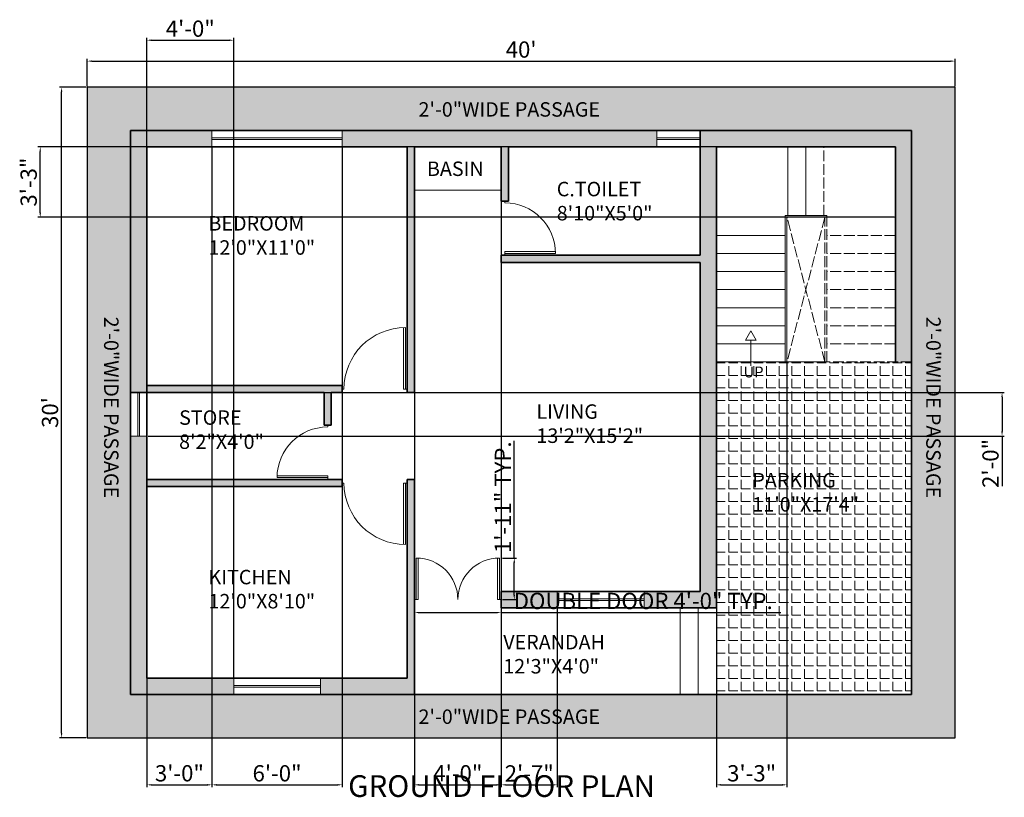
# Model space of a CAD drawing. Units: inches. Extents: x 1947 to 4744, y 610 to 1869.
# Tile 2 of 8: x 1947 to 2492, y 1428 to 1858. Entities that reach past the tile are written whole.
import ezdxf

# ---------------------------------------------------------------- set-up
doc = ezdxf.new("R2010")
doc.units = ezdxf.units.IN
doc.linetypes.add('ACAD_ISO02W100', pattern=[15, 12, -3])
for name, color, linetype, lineweight in [('A-ANNO-DIMS', 2, 'Continuous', 18), ('A-ANNO-SYMB', 2, 'Continuous', 18), ('A-ANNO-TEXT', 7, 'Continuous', 18), ('A-ANNO-TITL', 7, 'Continuous', 35), ('A-AREA-IDEN', 7, 'Continuous', 18), ('A-DOOR', 3, 'Continuous', 18), ('A-FLOR-FIXT', 9, 'Continuous', 18), ('A-FLOR-STRS', 7, 'Continuous', 18), ('A-FLOR-STRS-OVHD', 7, 'ACAD_ISO02W100', 13), ('A-GLAZ', 4, 'Continuous', 18), ('A-WALL', 7, 'Continuous', 35), ('C-PROP', 8, 'Continuous', 25)]:
    doc.layers.add(name, color=color, linetype=linetype, lineweight=lineweight)
doc.layers.add('A-FLOR-PATT', color=251, linetype='Continuous', lineweight=13, true_color=0x636466)
doc.layers.add('A-WALL-PATT', color=18, linetype='Continuous', lineweight=13, true_color=0x000000)
doc.styles.get("Standard").update_dxf_attribs({"font": 'arial.ttf'})
doc.dimstyles.new('ISO-25', dxfattribs={"dimtxt": 9, "dimasz": 2.5, "dimexe": 1.25, "dimexo": 0.625, "dimtad": 1, "dimdec": 1, "dimlunit": 3, "dimtxsty": 'Standard', "dimcen": 2.5, "dimadec": 0, "dimazin": 0, "dimtfac": 1, "dimtdec": 1, "dimtmove": 0, "dimatfit": 3, "dimfxl": 1, "dimarcsym": 0})
pattern_1 = [(0, (-1704.723, -21.7476), (0, 6.985), [5.08, -1.905]), (90, (-1704.723, -21.7476), (-6.985, 4e-16), [5.08, -1.905])]

# ---------------------------------------------------------------- blocks, each defined once
blk = doc.blocks.new('1')
for p, q in [((4267.36, 1627.82), (4267.36, 1650.82)), ((4268.36, 1627.82), (4268.36, 1650.82)), ((4312.36, 1627.82), (4312.36, 1650.82)), ((4313.36, 1627.82), (4313.36, 1650.82)), ((4266.36, 1627.82), (4268.36, 1627.82)), ((4314.36, 1627.82), (4312.36, 1627.82))]:
    blk.add_line(p, q)
at = {"ltscale": 0.5}
for centre, start, end in [((4267.36, 1627.82), 0, 90), ((4313.36, 1627.82), 90, 180)]:
    blk.add_arc(centre, 23, start, end, dxfattribs=at)
blk = doc.blocks.new('2')
for p, q in [((4319.45, 1679.18), (4319.45, 1713.18)), ((4320.45, 1679.18), (4320.45, 1713.18)), ((4318.45, 1679.18), (4320.45, 1679.18)), ((4353.45, 1679.18), (4354.45, 1679.18))]:
    blk.add_line(p, q)
at = {"ltscale": 0.5}
blk.add_arc((4319.45, 1679.18), 34, 0, 90, dxfattribs=at)
blk = doc.blocks.new('4')
for p, q in [((3808.6, 1693.11), (3808.6, 1721.11)), ((3809.6, 1693.11), (3809.6, 1721.11)), ((3807.6, 1693.11), (3809.6, 1693.11)), ((3836.6, 1693.11), (3837.6, 1693.11))]:
    blk.add_line(p, q)
at = {"ltscale": 0.5}
blk.add_arc((3808.6, 1693.11), 28, 0, 90, dxfattribs=at)
blk = doc.blocks.new('*D64')
at = {"layer": 'A-ANNO-DIMS', "color": 0, "lineweight": -2, "transparency": 16777216}
for p, q in [((1984.18, 1821.08), (1969.39, 1821.08)), ((1970.64, 1463.58), (1970.64, 1818.58)), ((1984.18, 1461.08), (1969.39, 1461.08))]:
    blk.add_line(p, q, dxfattribs=at)
at = {"layer": 'A-ANNO-DIMS', "color": 0, "transparency": 16777216}
for points in [[(1970.22, 1818.58), (1971.05, 1818.58), (1970.64, 1821.08)], [(1970.22, 1463.58), (1971.05, 1463.58), (1970.64, 1461.08)]]:
    blk.add_solid(points, dxfattribs=at)
at = {"layer": 'Defpoints', "color": 0, "transparency": 16777216}
for p in [(1970.64, 1821.08), (1984.81, 1821.08), (1984.81, 1461.08)]:
    blk.add_point(p, dxfattribs=at)
at = {"layer": 'A-ANNO-DIMS', "color": 0, "transparency": 16777216, "insert": (1965.41, 1641.08), "char_height": 9, "attachment_point": 5, "rotation": 90}
blk.add_mtext("30'", dxfattribs=at)
blk = doc.blocks.new('*D65')
at = {"layer": 'A-ANNO-DIMS', "color": 0, "lineweight": -2, "transparency": 16777216}
for p, q in [((1984.81, 1821.71), (1984.81, 1836.77)), ((1987.31, 1835.52), (2462.31, 1835.52)), ((2464.81, 1821.71), (2464.81, 1836.77))]:
    blk.add_line(p, q, dxfattribs=at)
at = {"layer": 'A-ANNO-DIMS', "color": 0, "transparency": 16777216}
for points in [[(1987.31, 1835.93), (1987.31, 1835.1), (1984.81, 1835.52)], [(2462.31, 1835.93), (2462.31, 1835.1), (2464.81, 1835.52)]]:
    blk.add_solid(points, dxfattribs=at)
at = {"layer": 'Defpoints', "color": 0, "transparency": 16777216}
for p in [(2464.81, 1835.52), (1984.81, 1821.08), (2464.81, 1821.08)]:
    blk.add_point(p, dxfattribs=at)
at = {"layer": 'A-ANNO-DIMS', "color": 0, "transparency": 16777216, "insert": (2224.81, 1840.74), "char_height": 9, "attachment_point": 5}
blk.add_mtext("40'", dxfattribs=at)
blk = doc.blocks.new('STAIR-DIRECTION')
blk.add_line((2.91, 14.18), (2.91, 0))
blk.add_lwpolyline([(2.91, 19.23), (0, 14.18), (5.83, 14.18)], close=True)
blk = doc.blocks.new('*D78')
at = {"layer": 'A-ANNO-DIMS', "color": 0, "lineweight": -2, "transparency": 16777216}
for p, q in [((2165.81, 1536.96), (2165.81, 1529.13)), ((2213.81, 1536.96), (2213.81, 1529.13)), ((2168.31, 1530.38), (2211.31, 1530.38)), ((2213.81, 1530.38), (2368.38, 1530.38))]:
    blk.add_line(p, q, dxfattribs=at)
at = {"layer": 'A-ANNO-DIMS', "color": 0, "transparency": 16777216}
for points in [[(2168.31, 1530.8), (2168.31, 1529.96), (2165.81, 1530.38)], [(2211.31, 1530.8), (2211.31, 1529.96), (2213.81, 1530.38)]]:
    blk.add_solid(points, dxfattribs=at)
at = {"layer": 'Defpoints', "color": 0, "transparency": 16777216}
for p in [(2165.81, 1537.58), (2213.81, 1537.58), (2213.81, 1530.38)]:
    blk.add_point(p, dxfattribs=at)
at = {"layer": 'A-ANNO-DIMS', "color": 0, "transparency": 16777216, "insert": (2292.34, 1535.66), "char_height": 9, "attachment_point": 5}
blk.add_mtext('DOUBLE DOOR 4\'-0" TYP.', dxfattribs=at)
blk = doc.blocks.new('*D79')
at = {"layer": 'A-ANNO-DIMS', "color": 0, "lineweight": -2, "transparency": 16777216}
for p, q in [((2221.01, 1560.58), (2221.01, 1625.33)), ((2214.43, 1560.58), (2222.26, 1560.58)), ((2221.01, 1540.08), (2221.01, 1558.08)), ((2214.43, 1537.58), (2222.26, 1537.58))]:
    blk.add_line(p, q, dxfattribs=at)
at = {"layer": 'A-ANNO-DIMS', "color": 0, "transparency": 16777216}
for points in [[(2220.59, 1558.08), (2221.42, 1558.08), (2221.01, 1560.58)], [(2220.59, 1540.08), (2221.42, 1540.08), (2221.01, 1537.58)]]:
    blk.add_solid(points, dxfattribs=at)
at = {"layer": 'Defpoints', "color": 0, "transparency": 16777216}
for p in [(2213.81, 1560.58), (2221.01, 1560.58), (2213.81, 1537.58)]:
    blk.add_point(p, dxfattribs=at)
at = {"layer": 'A-ANNO-DIMS', "color": 0, "transparency": 16777216, "insert": (2215.86, 1594.21), "char_height": 9, "attachment_point": 5, "rotation": 90}
blk.add_mtext('1\'-11" TYP.', dxfattribs=at)
blk = doc.blocks.new('*D96')
at = {"layer": 'A-ANNO-DIMS', "color": 0, "lineweight": -2, "transparency": 16777216}
for p, q in [((2332.81, 1668.46), (2332.81, 1433.83)), ((2371.81, 1668.46), (2371.81, 1433.83)), ((2335.31, 1435.08), (2369.31, 1435.08))]:
    blk.add_line(p, q, dxfattribs=at)
at = {"layer": 'A-ANNO-DIMS', "color": 0, "transparency": 16777216}
for points in [[(2335.31, 1435.5), (2335.31, 1434.66), (2332.81, 1435.08)], [(2369.31, 1435.5), (2369.31, 1434.66), (2371.81, 1435.08)]]:
    blk.add_solid(points, dxfattribs=at)
at = {"layer": 'Defpoints', "color": 0, "transparency": 16777216}
for p in [(2332.81, 1669.08), (2371.81, 1669.08), (2371.81, 1435.08)]:
    blk.add_point(p, dxfattribs=at)
at = {"layer": 'A-ANNO-DIMS', "color": 0, "transparency": 16777216, "insert": (2352.31, 1440.3), "char_height": 9, "attachment_point": 5}
blk.add_mtext('3\'-3"', dxfattribs=at)
blk = doc.blocks.new('*D97')
at = {"layer": 'A-ANNO-DIMS', "color": 0, "lineweight": -2, "transparency": 16777216}
for p, q in [((2431.18, 1788.08), (1957.56, 1788.08)), ((1958.81, 1751.58), (1958.81, 1785.58)), ((2431.18, 1749.08), (1957.56, 1749.08))]:
    blk.add_line(p, q, dxfattribs=at)
at = {"layer": 'A-ANNO-DIMS', "color": 0, "transparency": 16777216}
for points in [[(1958.39, 1785.58), (1959.22, 1785.58), (1958.81, 1788.08)], [(1958.39, 1751.58), (1959.22, 1751.58), (1958.81, 1749.08)]]:
    blk.add_solid(points, dxfattribs=at)
at = {"layer": 'Defpoints', "color": 0, "transparency": 16777216}
for p in [(1958.81, 1788.08), (2431.81, 1788.08), (2431.81, 1749.08)]:
    blk.add_point(p, dxfattribs=at)
at = {"layer": 'A-ANNO-DIMS', "color": 0, "transparency": 16777216, "insert": (1953.58, 1768.58), "char_height": 9, "attachment_point": 5, "rotation": 90}
blk.add_mtext('3\'-3"', dxfattribs=at)
blk = doc.blocks.new('*D99')
at = {"layer": 'A-ANNO-DIMS', "color": 0, "lineweight": -2, "transparency": 16777216}
for p, q in [((2165.81, 1763.46), (2165.81, 1433.83)), ((2213.81, 1763.46), (2213.81, 1433.83)), ((2168.31, 1435.08), (2211.31, 1435.08))]:
    blk.add_line(p, q, dxfattribs=at)
at = {"layer": 'A-ANNO-DIMS', "color": 0, "transparency": 16777216}
for points in [[(2168.31, 1435.5), (2168.31, 1434.66), (2165.81, 1435.08)], [(2211.31, 1435.5), (2211.31, 1434.66), (2213.81, 1435.08)]]:
    blk.add_solid(points, dxfattribs=at)
at = {"layer": 'Defpoints', "color": 0, "transparency": 16777216}
for p in [(2165.81, 1764.08), (2213.81, 1764.08), (2213.81, 1435.08)]:
    blk.add_point(p, dxfattribs=at)
at = {"layer": 'A-ANNO-DIMS', "color": 0, "transparency": 16777216, "insert": (2189.81, 1440.3), "char_height": 9, "attachment_point": 5}
blk.add_mtext('4\'-0"', dxfattribs=at)
blk = doc.blocks.new('*D104')
at = {"layer": 'A-ANNO-DIMS', "color": 0, "lineweight": -2, "transparency": 16777216}
for p, q in [((2017.81, 1787.46), (2017.81, 1433.83)), ((2053.81, 1787.46), (2053.81, 1433.83)), ((2020.31, 1435.08), (2051.31, 1435.08))]:
    blk.add_line(p, q, dxfattribs=at)
at = {"layer": 'A-ANNO-DIMS', "color": 0, "transparency": 16777216}
for points in [[(2020.31, 1435.5), (2020.31, 1434.66), (2017.81, 1435.08)], [(2051.31, 1435.5), (2051.31, 1434.66), (2053.81, 1435.08)]]:
    blk.add_solid(points, dxfattribs=at)
at = {"layer": 'Defpoints', "color": 0, "transparency": 16777216}
for p in [(2017.81, 1788.08), (2053.81, 1788.08), (2053.81, 1435.08)]:
    blk.add_point(p, dxfattribs=at)
at = {"layer": 'A-ANNO-DIMS', "color": 0, "transparency": 16777216, "insert": (2035.81, 1440.3), "char_height": 9, "attachment_point": 5}
blk.add_mtext('3\'-0"', dxfattribs=at)
blk = doc.blocks.new('*D105')
at = {"layer": 'A-ANNO-DIMS', "color": 0, "lineweight": -2, "transparency": 16777216}
for p, q in [((2053.81, 1787.46), (2053.81, 1433.83)), ((2125.81, 1787.46), (2125.81, 1433.83)), ((2056.31, 1435.08), (2123.31, 1435.08))]:
    blk.add_line(p, q, dxfattribs=at)
at = {"layer": 'A-ANNO-DIMS', "color": 0, "transparency": 16777216}
for points in [[(2056.31, 1435.5), (2056.31, 1434.66), (2053.81, 1435.08)], [(2123.31, 1435.5), (2123.31, 1434.66), (2125.81, 1435.08)]]:
    blk.add_solid(points, dxfattribs=at)
at = {"layer": 'Defpoints', "color": 0, "transparency": 16777216}
for p in [(2053.81, 1788.08), (2125.81, 1788.08), (2125.81, 1435.08)]:
    blk.add_point(p, dxfattribs=at)
at = {"layer": 'A-ANNO-DIMS', "color": 0, "transparency": 16777216, "insert": (2089.81, 1440.3), "char_height": 9, "attachment_point": 5}
blk.add_mtext('6\'-0"', dxfattribs=at)
blk = doc.blocks.new('*D106')
at = {"layer": 'A-ANNO-DIMS', "color": 0, "lineweight": -2, "transparency": 16777216}
for p, q in [((2017.81, 1494.71), (2017.81, 1848.33)), ((2020.31, 1847.08), (2063.31, 1847.08)), ((2065.81, 1494.71), (2065.81, 1848.33))]:
    blk.add_line(p, q, dxfattribs=at)
at = {"layer": 'A-ANNO-DIMS', "color": 0, "transparency": 16777216}
for points in [[(2020.31, 1847.5), (2020.31, 1846.66), (2017.81, 1847.08)], [(2063.31, 1847.5), (2063.31, 1846.66), (2065.81, 1847.08)]]:
    blk.add_solid(points, dxfattribs=at)
at = {"layer": 'Defpoints', "color": 0, "transparency": 16777216}
for p in [(2065.81, 1847.08), (2017.81, 1494.08), (2065.81, 1494.08)]:
    blk.add_point(p, dxfattribs=at)
at = {"layer": 'A-ANNO-DIMS', "color": 0, "transparency": 16777216, "insert": (2041.81, 1852.3), "char_height": 9, "attachment_point": 5}
blk.add_mtext('4\'-0"', dxfattribs=at)
blk = doc.blocks.new('*D107')
at = {"layer": 'A-ANNO-DIMS', "color": 0, "lineweight": -2, "transparency": 16777216}
for p, q in [((2213.81, 1532.46), (2213.81, 1433.83)), ((2244.81, 1532.46), (2244.81, 1433.83)), ((2216.31, 1435.08), (2242.31, 1435.08))]:
    blk.add_line(p, q, dxfattribs=at)
at = {"layer": 'A-ANNO-DIMS', "color": 0, "transparency": 16777216}
for points in [[(2216.31, 1435.5), (2216.31, 1434.66), (2213.81, 1435.08)], [(2242.31, 1435.5), (2242.31, 1434.66), (2244.81, 1435.08)]]:
    blk.add_solid(points, dxfattribs=at)
at = {"layer": 'Defpoints', "color": 0, "transparency": 16777216}
for p in [(2213.81, 1533.08), (2244.81, 1533.08), (2244.81, 1435.08)]:
    blk.add_point(p, dxfattribs=at)
at = {"layer": 'A-ANNO-DIMS', "color": 0, "transparency": 16777216, "insert": (2229.31, 1440.22), "char_height": 9, "attachment_point": 5}
blk.add_mtext('2\'-7"', dxfattribs=at)
blk = doc.blocks.new('*D111')
at = {"layer": 'A-ANNO-DIMS', "color": 0, "lineweight": -2, "transparency": 16777216}
for p, q in [((2018.43, 1652.08), (2492.06, 1652.08)), ((2490.81, 1649.58), (2490.81, 1630.58)), ((2018.43, 1628.08), (2492.06, 1628.08)), ((2490.81, 1628.08), (2490.81, 1600.25))]:
    blk.add_line(p, q, dxfattribs=at)
at = {"layer": 'A-ANNO-DIMS', "color": 0, "transparency": 16777216}
for points in [[(2490.39, 1649.58), (2491.22, 1649.58), (2490.81, 1652.08)], [(2490.39, 1630.58), (2491.22, 1630.58), (2490.81, 1628.08)]]:
    blk.add_solid(points, dxfattribs=at)
at = {"layer": 'Defpoints', "color": 0, "transparency": 16777216}
for p in [(2017.81, 1652.08), (2017.81, 1628.08), (2490.81, 1628.08)]:
    blk.add_point(p, dxfattribs=at)
at = {"layer": 'A-ANNO-DIMS', "color": 0, "transparency": 16777216, "insert": (2485.59, 1612.92), "char_height": 9, "attachment_point": 5, "rotation": 90}
blk.add_mtext('2\'-0"', dxfattribs=at)

msp = doc.modelspace()

# ---------------------------------------------------------------- hatches: boundary and pattern name
at = {"layer": 'A-FLOR-PATT'}
h = msp.add_hatch(dxfattribs=at)
h.set_pattern_fill('ANGLE', color=256)
h.set_pattern_definition(pattern_1)
h.paths.add_polyline_path([(1984.81, 1821.08), (1984.81, 1461.08), (2464.81, 1461.08), (2464.81, 1821.08)])
h.paths.add_polyline_path([(2440.81, 1797.08), (2440.81, 1485.08), (2008.81, 1485.08), (2008.81, 1797.08)], flags=16)
h.paths.add_polyline_path([(2431.81, 1788.08), (2431.81, 1669.08), (2392.81, 1669.08), (2332.81, 1669.08), (2332.81, 1533.08), (2213.81, 1533.08), (2213.81, 1542.08), (2323.81, 1542.08), (2323.81, 1724.08), (2213.81, 1724.08), (2213.81, 1728.08), (2323.81, 1728.08), (2323.81, 1788.08), (2217.81, 1788.08), (2217.81, 1758.08), (2213.81, 1758.08), (2213.81, 1764.08), (2165.81, 1764.08), (2165.81, 1652.08), (2161.81, 1652.08), (2161.81, 1788.08), (2017.81, 1788.08), (2017.81, 1656.08), (2125.81, 1656.08), (2125.81, 1652.08), (2119.81, 1652.08), (2119.81, 1634.08), (2115.81, 1634.08), (2115.81, 1652.08), (2017.81, 1652.08), (2017.81, 1604.08), (2125.81, 1604.08), (2125.81, 1600.08), (2017.81, 1600.08), (2017.81, 1494.08), (2113.81, 1494.08), (2113.81, 1489.08), (2065.81, 1489.08), (2065.81, 1494.08), (2017.81, 1494.08), (2017.81, 1600.08), (2125.81, 1600.08), (2125.81, 1604.08), (2017.81, 1604.08), (2017.81, 1628.08), (2012.81, 1628.08), (2012.81, 1652.08), (2115.81, 1652.08), (2115.81, 1634.08), (2119.81, 1634.08), (2119.81, 1652.08), (2125.81, 1652.08), (2125.81, 1656.08), (2017.81, 1656.08), (2017.81, 1788.08), (2053.81, 1788.08), (2053.81, 1793.08), (2125.81, 1793.08), (2125.81, 1788.08), (2161.81, 1788.08), (2161.81, 1652.08), (2165.81, 1652.08), (2165.81, 1788.08), (2213.81, 1788.08), (2213.81, 1758.08), (2217.81, 1758.08), (2217.81, 1788.08), (2299.81, 1788.08), (2299.81, 1793.08), (2323.81, 1793.08), (2323.81, 1728.08), (2213.81, 1728.08), (2213.81, 1724.08), (2323.81, 1724.08), (2323.81, 1542.08), (2292.81, 1542.08), (2292.81, 1533.08), (2332.81, 1533.08), (2332.81, 1788.08)], flags=0)
h.paths.add_polyline_path([(2371.81, 1749.08), (2392.81, 1749.08), (2392.81, 1669.08), (2382.31, 1709.08), (2371.81, 1669.08)], flags=0)
h.paths.add_polyline_path([(2170.5, 1767.41), (2209.94, 1767.41), (2209.94, 1784.49), (2170.5, 1784.49)], flags=8)
h.paths.add_polyline_path([(2165.8, 1464.23), (2278.79, 1464.23), (2278.79, 1481.31), (2165.8, 1481.31)], flags=24)
h.paths.add_polyline_path([(1989.56, 1696.36), (1989.56, 1583.37), (2006.64, 1583.37), (2006.64, 1696.36)], flags=24)
h.paths.add_polyline_path([(2444.3, 1696.36), (2444.3, 1583.37), (2461.38, 1583.37), (2461.38, 1696.36)], flags=24)
h.paths.add_polyline_path([(2165.8, 1800.23), (2278.79, 1800.23), (2278.79, 1817.31), (2165.8, 1817.31)], flags=24)
h.paths.add_polyline_path([(2211.53, 1492.13), (2283.09, 1492.13), (2283.09, 1522.55), (2211.53, 1522.55)], flags=8)
h.paths.add_polyline_path([(2349.32, 1581.74), (2411.18, 1581.74), (2411.18, 1612.15), (2349.32, 1612.15)], flags=8)
h.paths.add_polyline_path([(2032.89, 1616.39), (2082.97, 1616.39), (2082.97, 1646.8), (2032.89, 1646.8)], flags=8)
h.paths.add_polyline_path([(2241.79, 1742.83), (2298.24, 1742.83), (2298.24, 1773.25), (2241.79, 1773.25)], flags=8)
h.paths.add_polyline_path([(2229.87, 1619.7), (2291.74, 1619.7), (2291.74, 1650.11), (2229.87, 1650.11)], flags=8)
h.paths.add_polyline_path([(2048.47, 1528.14), (2110.34, 1528.14), (2110.34, 1558.56), (2048.47, 1558.56)], flags=8)
h.paths.add_polyline_path([(2048.47, 1723.84), (2112.73, 1723.84), (2112.73, 1754.25), (2048.47, 1754.25)], flags=8)
h = msp.add_hatch(dxfattribs=at)
h.set_pattern_fill('ANGLE', color=256)
h.set_pattern_definition(pattern_1)
h.paths.add_polyline_path([(2440.81, 1669.08), (2392.81, 1669.08), (2332.81, 1669.08), (2332.81, 1533.08), (2332.81, 1485.08), (2440.81, 1485.08)])
h.paths.add_polyline_path([(2346.28, 1657.09), (2360.6, 1657.09), (2360.6, 1669.9), (2346.28, 1669.9)], flags=9)
h.paths.add_polyline_path([(2349.32, 1581.74), (2411.18, 1581.74), (2411.18, 1612.15), (2349.32, 1612.15)], flags=24)
at = {"layer": 'A-WALL-PATT'}
h = msp.add_hatch(color=256, dxfattribs=at)
h.dxf.hatch_style = 1
h.paths.add_polyline_path([(2053.81, 1788.08), (2053.81, 1797.08), (2008.81, 1797.08), (2008.81, 1652.08), (2115.81, 1652.08), (2115.81, 1634.08), (2119.81, 1634.08), (2119.81, 1652.08), (2125.81, 1652.08), (2125.81, 1656.08), (2017.81, 1656.08), (2017.81, 1788.08)])
h.paths.add_polyline_path([(2125.81, 1797.08), (2125.81, 1788.08), (2161.81, 1788.08), (2161.81, 1652.08), (2165.81, 1652.08), (2165.81, 1788.08), (2213.81, 1788.08), (2213.81, 1758.08), (2217.81, 1758.08), (2217.81, 1788.08), (2299.81, 1788.08), (2299.81, 1797.08)])
h.paths.add_polyline_path([(2323.81, 1728.08), (2213.81, 1728.08), (2213.81, 1724.08), (2323.81, 1724.08), (2323.81, 1542.08), (2292.81, 1542.08), (2292.81, 1533.08), (2332.81, 1533.08), (2332.81, 1788.08), (2431.81, 1788.08), (2431.81, 1669.08), (2440.81, 1669.08), (2440.81, 1797.08), (2323.81, 1797.08)])
h.paths.add_polyline_path([(2165.81, 1485.08), (2165.81, 1604.08), (2161.81, 1604.08), (2161.81, 1494.08), (2113.81, 1494.08), (2113.81, 1485.08)])
h.paths.add_polyline_path([(2017.81, 1494.08), (2017.81, 1600.08), (2125.81, 1600.08), (2125.81, 1604.08), (2017.81, 1604.08), (2017.81, 1628.08), (2008.81, 1628.08), (2008.81, 1485.08), (2065.81, 1485.08), (2065.81, 1494.08)])
h.paths.add_polyline_path([(2244.81, 1533.08), (2244.81, 1542.08), (2213.81, 1542.08), (2213.81, 1533.08)], flags=17)

# ---------------------------------------------------------------- linework, layer by layer
at = {"layer": 'A-FLOR-FIXT'}
msp.add_line((2213.81, 1764.08), (2165.81, 1764.08), dxfattribs=at)
at = {"layer": 'A-FLOR-STRS'}
for p, q in [((2372.31, 1750.08), (2372.31, 1788.08)), ((2382.31, 1750.08), (2382.31, 1788.08)), ((2370.81, 1749.08), (2332.81, 1749.08)), ((2393.81, 1750.08), (2370.81, 1750.08)), ((2370.81, 1669.08), (2370.81, 1750.08)), ((2392.81, 1749.08), (2371.81, 1749.08)), ((2371.81, 1669.08), (2371.81, 1749.08)), ((2370.81, 1739.08), (2332.81, 1739.08)), ((2370.81, 1729.08), (2332.81, 1729.08)), ((2370.81, 1719.08), (2332.81, 1719.08)), ((2370.81, 1709.08), (2332.81, 1709.08)), ((2370.81, 1699.08), (2332.81, 1699.08)), ((2370.81, 1689.08), (2332.81, 1689.08)), ((2370.81, 1679.08), (2332.81, 1679.08)), ((2392.81, 1669.08), (2332.81, 1669.08)), ((2312.81, 1533.08), (2312.81, 1485.08)), ((2322.81, 1533.08), (2322.81, 1485.08)), ((2332.81, 1533.08), (2332.81, 1485.08))]:
    msp.add_line(p, q, dxfattribs=at)
at = {"layer": 'A-FLOR-STRS-OVHD', "ltscale": 0.5}
for p, q in [((2392.31, 1750.08), (2392.31, 1788.08)), ((2392.81, 1749.08), (2371.81, 1669.08)), ((2392.81, 1669.08), (2371.81, 1749.08)), ((2392.81, 1669.08), (2392.81, 1749.08)), ((2393.81, 1669.08), (2393.81, 1750.08)), ((2431.81, 1749.08), (2393.81, 1749.08)), ((2431.81, 1739.08), (2393.81, 1739.08)), ((2431.81, 1729.08), (2393.81, 1729.08)), ((2431.81, 1719.08), (2393.81, 1719.08)), ((2431.81, 1709.08), (2393.81, 1709.08)), ((2431.81, 1699.08), (2393.81, 1699.08)), ((2431.81, 1689.08), (2393.81, 1689.08)), ((2431.81, 1679.08), (2393.81, 1679.08)), ((2440.81, 1669.08), (2392.81, 1669.08))]:
    msp.add_line(p, q, dxfattribs=at)
at = {"layer": 'A-GLAZ'}
for p, q in [((2053.81, 1788.08), (2053.81, 1797.08)), ((2125.81, 1793.08), (2053.81, 1793.08)), ((2125.81, 1792.08), (2053.81, 1792.08)), ((2125.81, 1788.08), (2125.81, 1797.08)), ((2299.81, 1788.08), (2299.81, 1797.08)), ((2323.81, 1793.08), (2299.81, 1793.08)), ((2323.81, 1792.08), (2299.81, 1792.08)), ((2012.81, 1652.08), (2012.81, 1628.08)), ((2013.81, 1652.08), (2013.81, 1628.08)), ((2017.81, 1628.08), (2008.81, 1628.08)), ((2244.81, 1533.08), (2244.81, 1542.08)), ((2292.81, 1533.08), (2292.81, 1542.08)), ((2292.81, 1538.08), (2244.81, 1538.08)), ((2292.81, 1537.08), (2244.81, 1537.08)), ((2065.81, 1485.08), (2065.81, 1494.08)), ((2113.81, 1485.08), (2113.81, 1494.08)), ((2113.81, 1490.08), (2065.81, 1490.08)), ((2113.81, 1489.08), (2065.81, 1489.08))]:
    msp.add_line(p, q, dxfattribs=at)
at = {"layer": 'A-WALL'}
for p, q in [((2440.81, 1797.08), (2008.81, 1797.08)), ((2008.81, 1797.08), (2008.81, 1485.08)), ((2323.81, 1728.08), (2323.81, 1797.08)), ((2440.81, 1485.08), (2440.81, 1797.08)), ((2161.81, 1788.08), (2017.81, 1788.08)), ((2017.81, 1788.08), (2017.81, 1656.08)), ((2161.81, 1788.08), (2161.81, 1652.08)), ((2213.81, 1788.08), (2165.81, 1788.08)), ((2165.81, 1788.08), (2165.81, 1652.08)), ((2213.81, 1758.08), (2213.81, 1788.08)), ((2323.81, 1788.08), (2217.81, 1788.08)), ((2217.81, 1758.08), (2217.81, 1788.08)), ((2431.81, 1788.08), (2332.81, 1788.08)), ((2332.81, 1533.08), (2332.81, 1788.08)), ((2431.81, 1669.08), (2431.81, 1788.08)), ((2217.81, 1758.08), (2213.81, 1758.08)), ((2323.81, 1728.08), (2213.81, 1728.08)), ((2213.81, 1724.08), (2213.81, 1728.08)), ((2213.81, 1724.08), (2323.81, 1724.08)), ((2323.81, 1542.08), (2323.81, 1724.08)), ((2125.81, 1656.08), (2017.81, 1656.08)), ((2125.81, 1656.08), (2125.81, 1652.08)), ((2115.81, 1652.08), (2008.81, 1652.08)), ((2017.81, 1652.08), (2017.81, 1604.08)), ((2115.81, 1652.08), (2115.81, 1634.08)), ((2125.81, 1652.08), (2119.81, 1652.08)), ((2119.81, 1652.08), (2119.81, 1634.08)), ((2165.81, 1652.08), (2161.81, 1652.08)), ((2119.81, 1634.08), (2115.81, 1634.08)), ((2125.81, 1604.08), (2017.81, 1604.08)), ((2125.81, 1604.08), (2125.81, 1600.08)), ((2165.81, 1604.08), (2161.81, 1604.08)), ((2161.81, 1604.08), (2161.81, 1494.08)), ((2165.81, 1604.08), (2165.81, 1485.08)), ((2125.81, 1600.08), (2017.81, 1600.08)), ((2017.81, 1600.08), (2017.81, 1494.08)), ((2213.81, 1542.08), (2213.81, 1533.08)), ((2213.81, 1542.08), (2323.81, 1542.08)), ((2213.81, 1533.08), (2332.81, 1533.08)), ((2017.81, 1494.08), (2161.81, 1494.08)), ((2008.81, 1485.08), (2440.81, 1485.08))]:
    msp.add_line(p, q, dxfattribs=at)
at = {"layer": 'C-PROP'}
msp.add_lwpolyline([(1984.81, 1461.08), (2464.81, 1461.08), (2464.81, 1821.08), (1984.81, 1821.08)], close=True, dxfattribs=at)

# ---------------------------------------------------------------- block references
at = {"layer": 'A-ANNO-SYMB'}
msp.add_blockref('STAIR-DIRECTION', (2348.89, 1667), dxfattribs=at)
at = {"layer": 'A-DOOR', "xscale": -1, "rotation": 270}
msp.add_blockref('4', (522.7, -2079.52), dxfattribs=at)
at = {"layer": 'A-DOOR', "xscale": -1}
msp.add_blockref('2', (6480.26, -25.1), dxfattribs=at)
at = {"layer": 'A-DOOR'}
for name, p, rotation in [('4', (3810.92, -2203.52), 90), ('2', (6480.26, 3281.26), 180)]:
    msp.add_blockref(name, p, dxfattribs=dict(at, rotation=rotation))
msp.add_blockref('1', (-2100.55, -90.24), dxfattribs=at)

# ---------------------------------------------------------------- texts
at = {"layer": 'A-ANNO-TEXT', "attachment_point": 1}
for s, insert, char_height in [('{\\fTimes New Roman|b0|i0|c0|p18;BASIN}', (2172.7, 1779.96), 8), ('{\\fTimes New Roman|b0|i0|c0|p18;UP}', (2347.83, 1666.5), 6)]:
    msp.add_mtext_dynamic_manual_height_columns(s, width=158.3328, gutter_width=12.5, heights=[0], dxfattribs=dict(at, insert=insert, char_height=char_height))
at = {"layer": 'A-ANNO-TITL', "insert": (2129.11, 1440.38), "char_height": 12, "attachment_point": 1}
msp.add_mtext_dynamic_manual_height_columns('{\\fTimes New Roman|b0|i0|c0|p18;GROUND FLOOR PLAN}', width=253.4596, gutter_width=12.5, heights=[0], dxfattribs=at)
at = {"layer": 'A-AREA-IDEN', "char_height": 8, "attachment_point": 1}
for s, width, heights, insert in [('{\\fTimes New Roman|b0|i0|c0|p18;2\'-0"WIDE PASSAGE}', 158.3328, [0], (2168.05, 1812.78)), ('{\\fTimes New Roman|b0|i0|c0|p18;C.TOILET\\P8\'10"X5\'0"}', 64.3566, [21.47], (2244.5, 1768.72)), ('{\\fTimes New Roman|b0|i0|c0|p18;BEDROOM\\P12\'0"X11\'0"}', 64.3566, [0], (2051.86, 1749.73)), ('{\\fTimes New Roman|b0|i0|c0|p18;LIVING\\P13\'2"X15\'2"}', 64.3566, [21.47], (2233.26, 1645.59)), ('{\\fTimes New Roman|b0|i0|c0|p18;STORE\\P8\'2"X4\'0"}', 64.3566, [21.47], (2035.63, 1642.28)), ('{\\fTimes New Roman|b0|i0|c0|p18;PARKING\\P11\'0"X17\'4"}', 64.3566, [0], (2352.7, 1607.62)), ('{\\fTimes New Roman|b0|i0|c0|p18;KITCHEN\\P12\'0"X8\'10"}', 64.3566, [0], (2051.86, 1554.03)), ('{\\fTimes New Roman|b0|i0|c0|p18;VERANDAH\\P12\'3"X4\'0"}', 64.3566, [0], (2214.92, 1518.02)), ('{\\fTimes New Roman|b0|i0|c0|p18;2\'-0"WIDE PASSAGE}', 158.3328, [0], (2168.05, 1476.78))]:
    msp.add_mtext_dynamic_manual_height_columns(s, width=width, gutter_width=12.5, heights=heights, dxfattribs=dict(at, insert=insert))
at = {"layer": 'A-AREA-IDEN', "char_height": 8, "attachment_point": 1, "rotation": 270}
for insert in [(2002.12, 1694.11), (2456.86, 1694.11)]:
    msp.add_mtext_dynamic_manual_height_columns('{\\fTimes New Roman|b0|i0|c0|p18;2\'-0"WIDE PASSAGE}', width=158.3328, gutter_width=12.5, heights=[0], dxfattribs=dict(at, insert=insert))

# ---------------------------------------------------------------- dimensions: what is measured, and where the dimension line sits
at = {"layer": 'A-ANNO-DIMS'}
for base, p1, p2, override, picture, middle in [((2065.81, 1847.08), (2017.81, 1494.08), (2065.81, 1494.08), {"dimdec": 1, "dimlfac": 1, "dimrnd": 0, "dimzin": 1, "dimdsep": 46, "dimlunit": 4, "dimfrac": 2}, '*D106', (2041.81, 1852.3)), ((2464.81, 1835.52), (1984.81, 1821.08), (2464.81, 1821.08), {"dimclrd": 0, "dimclre": 0, "dimclrt": 0}, '*D65', (2224.81, 1840.74)), ((2053.81, 1435.08), (2017.81, 1788.08), (2053.81, 1788.08), {"dimdec": 1, "dimlfac": 1, "dimrnd": 0, "dimzin": 1, "dimdsep": 46, "dimlunit": 4, "dimfrac": 2}, '*D104', (2035.81, 1440.3)), ((2125.81, 1435.08), (2053.81, 1788.08), (2125.81, 1788.08), {"dimdec": 1, "dimlfac": 1, "dimrnd": 0, "dimzin": 1, "dimdsep": 46, "dimlunit": 4, "dimfrac": 2}, '*D105', (2089.81, 1440.3)), ((2213.81, 1435.08), (2165.81, 1764.08), (2213.81, 1764.08), {"dimdec": 1, "dimlfac": 1, "dimrnd": 0, "dimzin": 1, "dimdsep": 46, "dimlunit": 4, "dimfrac": 2}, '*D99', (2189.81, 1440.3)), ((2371.81, 1435.08), (2332.81, 1669.08), (2371.81, 1669.08), {"dimdec": 1, "dimlfac": 1, "dimrnd": 0, "dimzin": 1, "dimdsep": 46, "dimlunit": 4, "dimfrac": 2}, '*D96', (2352.31, 1440.3)), ((2244.81, 1435.08), (2213.81, 1533.08), (2244.81, 1533.08), {"dimdec": 1, "dimlfac": 1, "dimrnd": 0, "dimzin": 1, "dimdsep": 46, "dimlunit": 4, "dimfrac": 2}, '*D107', (2229.31, 1440.22))]:
    dim = msp.add_linear_dim(base=base, p1=p1, p2=p2, dimstyle='ISO-25', override=override, dxfattribs=at)
    dim.commit()
    dim.dimension.update_dxf_attribs({"geometry": picture, "text_midpoint": middle})
for base, p1, p2, override, picture, middle in [((1970.64, 1821.08), (1984.81, 1461.08), (1984.81, 1821.08), {"dimclrd": 0, "dimclre": 0, "dimclrt": 0}, '*D64', (1965.41, 1641.08)), ((1958.81, 1788.08), (2431.81, 1749.08), (2431.81, 1788.08), {"dimdec": 1, "dimlfac": 1, "dimrnd": 0, "dimzin": 1, "dimdsep": 46, "dimlunit": 4, "dimfrac": 2}, '*D97', (1953.58, 1768.58)), ((2490.81, 1628.08), (2017.81, 1652.08), (2017.81, 1628.08), {"dimdec": 1, "dimlfac": 1, "dimrnd": 0, "dimzin": 1, "dimdsep": 46, "dimlunit": 4, "dimfrac": 2}, '*D111', (2485.59, 1612.92))]:
    dim = msp.add_linear_dim(base=base, p1=p1, p2=p2, angle=90, dimstyle='ISO-25', override=override, dxfattribs=at)
    dim.commit()
    dim.dimension.update_dxf_attribs({"geometry": picture, "text_midpoint": middle})
dim = msp.add_linear_dim(base=(2221.01, 1560.58), p1=(2213.81, 1537.58), p2=(2213.81, 1560.58), angle=90, text='<> TYP.', dimstyle='ISO-25', override={"dimdec": 1, "dimlfac": 1, "dimrnd": 0, "dimzin": 1, "dimdsep": 46, "dimlunit": 4, "dimfrac": 2}, dxfattribs=at)
dim.commit()
dim.dimension.update_dxf_attribs({"geometry": '*D79', "text_midpoint": (2215.86, 1594.21)})
dim = msp.add_linear_dim(base=(2213.81, 1530.38), p1=(2165.81, 1537.58), p2=(2213.81, 1537.58), text='DOUBLE DOOR <> TYP.', dimstyle='ISO-25', override={"dimdec": 1, "dimlfac": 1, "dimrnd": 0, "dimzin": 1, "dimdsep": 46, "dimlunit": 4, "dimfrac": 2}, dxfattribs=at)
dim.commit()
dim.dimension.update_dxf_attribs({"geometry": '*D78', "text_midpoint": (2292.34, 1535.66)})

doc.saveas('drawing.dxf')
